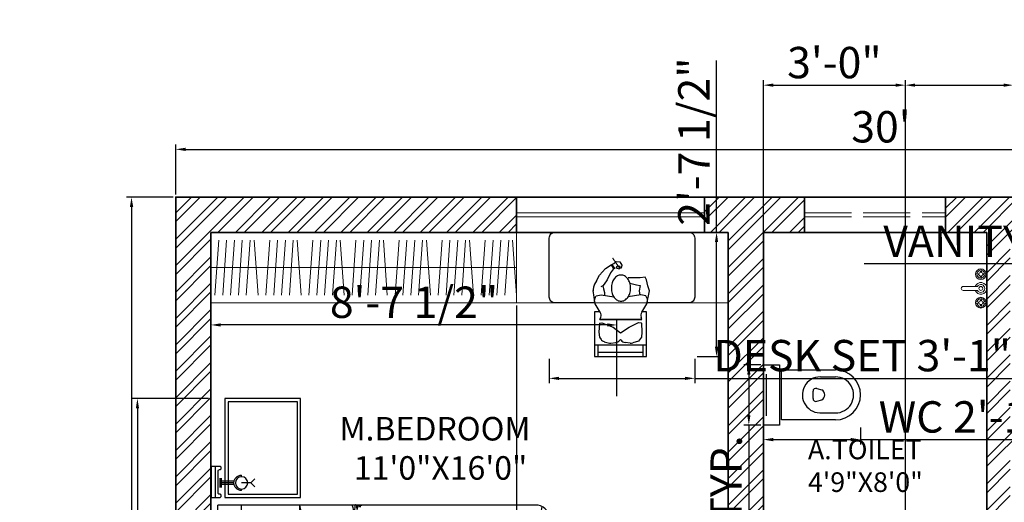
# Model space of a CAD drawing. Units: inches. Extents: x 3595 to 4516, y 2363 to 2965.
# Tile 11 of 12: x 4041 to 4293, y 2825 to 2948. Entities that reach past the tile are written whole.
import ezdxf

# ---------------------------------------------------------------- set-up
doc = ezdxf.new("R2010")
doc.units = ezdxf.units.IN
doc.linetypes.add('ACAD_ISO02W100', pattern=[15, 12, -3])
for name, color, linetype, lineweight in [('A-ANNO-DIMS', 2, 'Continuous', 18), ('A-AREA-IDEN', 7, 'Continuous', 18), ('A-FLOR-CASE', 9, 'Continuous', 18), ('A-FLOR-FIXT', 8, 'Continuous', 18), ('A-FURN', 43, 'Continuous', 18), ('A-GLAZ', 4, 'Continuous', 18), ('A-GLAZ-HIGH', 4, 'ACAD_ISO02W100', 18), ('A-WALL', 7, 'Continuous', 35)]:
    doc.layers.add(name, color=color, linetype=linetype, lineweight=lineweight)
doc.layers.add('A-WALL-PATT', color=251, linetype='Continuous', lineweight=13, true_color=0x636466)
for name, color, linetype in [('CEIL', 4, 'Continuous'), ('ELEC', 4, 'Continuous'), ('FUR', 42, 'Continuous'), ('NOITHAT', 21, 'Continuous'), ('SANTEH', 7, 'Continuous'), ('wood', 26, 'Continuous')]:
    doc.layers.add(name, color=color, linetype=linetype)
doc.styles.get("Standard").update_dxf_attribs({"font": 'arial.ttf'})
doc.dimstyles.new('ISO-25', dxfattribs={"dimtxt": 8, "dimasz": 2.5, "dimexe": 1.25, "dimexo": 0.625, "dimtad": 1, "dimdec": 1, "dimlunit": 3, "dimtxsty": 'Standard', "dimcen": 2.5, "dimadec": 0, "dimazin": 0, "dimtfac": 1, "dimtdec": 1, "dimtmove": 0, "dimatfit": 3, "dimfxl": 1, "dimarcsym": 0})

# ---------------------------------------------------------------- blocks, each defined once
blk = doc.blocks.new('*D5')
at = {"layer": 'A-ANNO-DIMS', "color": 0, "lineweight": -2, "transparency": 16777216}
for p, q in [((4081.24, 2903.67), (4081.24, 2916.47)), ((4441.24, 2903.67), (4441.24, 2916.47)), ((4083.74, 2915.22), (4438.74, 2915.22))]:
    blk.add_line(p, q, dxfattribs=at)
at = {"layer": 'A-ANNO-DIMS', "color": 0, "transparency": 16777216}
for points in [[(4083.74, 2915.63), (4083.74, 2914.8), (4081.24, 2915.22)], [(4438.74, 2915.63), (4438.74, 2914.8), (4441.24, 2915.22)]]:
    blk.add_solid(points, dxfattribs=at)
at = {"layer": 'Defpoints', "color": 0, "transparency": 16777216}
for p in [(4441.24, 2915.22), (4081.24, 2903.04), (4441.24, 2903.04)]:
    blk.add_point(p, dxfattribs=at)
at = {"layer": 'A-ANNO-DIMS', "color": 0, "transparency": 16777216, "insert": (4261.24, 2919.93), "char_height": 8, "attachment_point": 5}
blk.add_mtext("30'", dxfattribs=at)
blk = doc.blocks.new('*D6')
at = {"layer": 'A-ANNO-DIMS', "color": 0, "lineweight": -2, "transparency": 16777216}
for p, q in [((4080.62, 2903.04), (4068.71, 2903.04)), ((4069.96, 2900.54), (4069.96, 2401.54)), ((4080.62, 2399.04), (4068.71, 2399.04))]:
    blk.add_line(p, q, dxfattribs=at)
at = {"layer": 'A-ANNO-DIMS', "color": 0, "transparency": 16777216}
for points in [[(4069.55, 2900.54), (4070.38, 2900.54), (4069.96, 2903.04)], [(4069.55, 2401.54), (4070.38, 2401.54), (4069.96, 2399.04)]]:
    blk.add_solid(points, dxfattribs=at)
at = {"layer": 'Defpoints', "color": 0, "transparency": 16777216}
for p in [(4081.24, 2903.04), (4069.96, 2399.04), (4081.24, 2399.04)]:
    blk.add_point(p, dxfattribs=at)
at = {"layer": 'A-ANNO-DIMS', "color": 0, "transparency": 16777216, "insert": (4065.32, 2651.04), "char_height": 8, "attachment_point": 5, "rotation": 90}
blk.add_mtext("42'", dxfattribs=at)
blk = doc.blocks.new('*X14')
at = {"color": 0}
for p, q in [((3155.9, 8182.9), (3155.9, 8182.9)), ((3147.8, 8143.4), (3147.8, 8143.4)), ((3283, 8049.6), (3283, 8049.6)), ((3209.5, 8023.9), (3209.5, 8023.9)), ((3251.6, 7997), (3251.6, 7997)), ((3154.1, 7950.7), (3154.1, 7950.7))]:
    blk.add_line(p, q, dxfattribs=at)
blk = doc.blocks.new('*X13')
at = {"color": 0}
for p, q in [((3155.9, 8182.9), (3155.9, 8182.9)), ((3139.8, 7939.7), (3139.8, 7939.7))]:
    blk.add_line(p, q, dxfattribs=at)
blk = doc.blocks.new('*X12')
at = {"color": 0}
for p, q in [((3155.9, 8182.9), (3155.9, 8182.9)), ((3139.8, 7939.7), (3139.8, 7939.7))]:
    blk.add_line(p, q, dxfattribs=at)
blk = doc.blocks.new('*X11')
at = {"color": 0}
for p, q in [((3163, 7776.2), (3163, 7776.2)), ((3422.2, 7761.3), (3422.2, 7761.3)), ((3236.2, 7675.7), (3236.2, 7675.7)), ((3244.3, 7698.6), (3244.3, 7698.6)), ((3340.3, 7689.4), (3340.3, 7689.4))]:
    blk.add_line(p, q, dxfattribs=at)
blk = doc.blocks.new('BED1')
for p, q in [((0, -1000), (0, 800)), ((150, 800), (0, 800)), ((150, 800), (150, -1000)), ((2058.7, 800), (150, 800)), ((528, 800), (528, -1000)), ((211.8, 614.9), (277.5, 585.4)), ((2537.2, 404.9), (2237.2, 404.9)), ((2187.2, 354.9), (2187.2, -545.1)), ((2587.2, -545.1), (2587.2, 354.9)), ((2566.3, 178.5), (2565.2, 177.4)), ((2582, 188.1), (2565.4, 174.8)), ((2565.4, 174.8), (2585.7, 165.4)), ((2566.3, -296.8), (2565.2, -297.9)), ((2582, -287.1), (2565.4, -300.5)), ((2565.4, -300.5), (2585.7, -309.9)), ((2237.2, -595.1), (2537.2, -595.1)), ((150, -1000), (0, -1000)), ((150, -1000), (2063.5, -1000))]:
    blk.add_line(p, q)
for points in [[(934, 797.9), (930.9, 797.7), (928.3, 797.4), (926.3, 796.9), (924.9, 796.3), (923.8, 795.6), (923.1, 794.8), (922.7, 793.8), (922.5, 792.7), (922.4, 791.5), (922.5, 790.3), (922.6, 789.2), (922.6, 788.3), (922.6, 787.6), (922.4, 787.3), (922, 787.4), (921.4, 787.9), (920.6, 788.9), (919.5, 790.2), (918.4, 791.6), (917.1, 793.1), (915.9, 794.6), (914.6, 796), (913.3, 797.1), (912.2, 797.9), (911.1, 798.3), (910.1, 798.4), (909.2, 798), (908.3, 797.1), (907.5, 795.8), (906.8, 793.9), (906, 791.4), (905.4, 788.5), (904.8, 785.2), (904.2, 781.7), (903.7, 778.4), (903.2, 775.4), (902.8, 772.9), (902.5, 771.3), (902.3, 770.6), (902.1, 771.2), (902, 772.8), (901.8, 775.2), (901.7, 778.1), (901.5, 781.5), (901.2, 785), (900.8, 788.4), (900.2, 791.5), (899.5, 794.1), (898.6, 796.2), (897.6, 797.9), (896.5, 799.2), (895.3, 800), (894.1, 800.5), (893, 800.7), (891.9, 800.5), (890.9, 800.1), (890, 799), (889.1, 797.1), (888.3, 794), (887.6, 789.3), (886.9, 782.9), (886.2, 774.2), (885.5, 763.1), (884.8, 749.5), (884.2, 734.2), (883.6, 718.3), (883, 702.8), (882.5, 688.8), (882, 677.5), (881.7, 669.8), (881.5, 666.9), (881.3, 669.4), (881.3, 676.7), (881.3, 687.8), (881.2, 701.5), (881.1, 716.8), (880.8, 732.6), (880.2, 748), (879.4, 761.8), (878.3, 773.2), (876.9, 782.2), (875.1, 789.2), (872.9, 794.4), (870.3, 798), (869, 799)], [(2150, -913.5), (2150, 723.2)], [(2327.6, 182.3), (2530, 185.9), (2550.8, 181.9), (2561.7, 179), (2566, 176.7), (2566.9, 174.4), (2566.3, 171.9), (2562, 169.2), (2550.3, 166.5), (2527.7, 163.9), (2490.6, 161.8), (2345.5, 160.2), (2317.8, 158.5)], [(494.7, 3.1), (458.9, 95.3)], [(2149.7, -259.9), (2150, -268.4), (2150.1, -274.1), (2150.1, -278.1), (2150, -281.4), (2149.8, -284), (2149.5, -286.1), (2149.1, -287.8), (2148.7, -289), (2148.1, -289.9), (2147.4, -290.5), (2146.6, -290.8), (2145.6, -291), (2144.6, -291), (2143.6, -291), (2142.7, -290.9), (2141.9, -290.9), (2141.4, -290.9), (2141.1, -291), (2141.2, -291.4), (2141.7, -291.9), (2142.5, -292.6), (2143.5, -293.4), (2144.7, -294.4), (2146, -295.4), (2147.2, -296.5), (2148.4, -297.6), (2149.3, -298.6), (2150, -299.6), (2150.3, -300.5), (2150.4, -301.3), (2150, -302.1), (2149.3, -302.8), (2148.2, -303.5), (2146.6, -304.1), (2144.6, -304.7), (2142.1, -305.2), (2139.3, -305.7), (2136.5, -306.2), (2133.7, -306.6), (2131.2, -307), (2129.2, -307.3), (2127.8, -307.6), (2127.3, -307.8), (2127.7, -308), (2129, -308.1), (2131, -308.2), (2133.5, -308.3), (2136.3, -308.5), (2139.2, -308.7), (2142, -309), (2144.6, -309.5), (2146.8, -310.1), (2148.6, -310.9), (2150, -311.7), (2151, -312.7), (2151.7, -313.6), (2152.1, -314.6), (2152.3, -315.6), (2152.2, -316.5), (2151.8, -317.3), (2150.9, -318.1), (2149.3, -318.8), (2146.7, -319.4), (2142.8, -320), (2137.4, -320.6), (2130.2, -321.2), (2121, -321.8), (2109.7, -322.3), (2096.9, -322.9), (2083.6, -323.4), (2070.7, -323.9), (2059.1, -324.3), (2049.6, -324.7), (2043.2, -325), (2040.8, -325.2), (2042.9, -325.3), (2049, -325.3), (2058.2, -325.3), (2069.6, -325.4), (2082.3, -325.5), (2095.6, -325.8), (2108.4, -326.2), (2119.9, -326.8), (2129.4, -327.8), (2136.9, -329), (2142.7, -330.5), (2147, -332.3), (2150, -334.4), (2150.9, -335.6)], [(2246.5, -294.4), (2530, -289.4), (2550.8, -293.4), (2561.7, -296.3), (2566, -298.6), (2566.9, -300.8), (2566.3, -303.4), (2562, -306.1), (2550.3, -308.8), (2527.7, -311.3), (2490.6, -313.5), (2345.5, -315), (2238.6, -321.8)], [(1733.7, -998.3), (1731.1, -998.1), (1729, -997.8), (1727.4, -997.4), (1726.1, -997), (1725.2, -996.4), (1724.7, -995.7), (1724.3, -994.8), (1724.1, -993.9), (1724.1, -992.9), (1724.1, -991.9), (1724.2, -991), (1724.2, -990.2), (1724.2, -989.7), (1724.1, -989.4), (1723.8, -989.5), (1723.2, -990), (1722.5, -990.8), (1721.7, -991.8), (1720.7, -993), (1719.7, -994.3), (1718.6, -995.5), (1717.5, -996.6), (1716.5, -997.6), (1715.5, -998.3), (1714.6, -998.6), (1713.8, -998.6), (1713, -998.3), (1712.3, -997.6), (1711.7, -996.5), (1711, -994.9), (1710.4, -992.9), (1709.9, -990.4), (1709.4, -987.6), (1708.9, -984.8), (1708.5, -982), (1708.1, -979.5), (1707.8, -977.4), (1707.5, -976.1), (1707.3, -975.5), (1707.1, -976), (1707, -977.3), (1706.9, -979.3), (1706.8, -981.8), (1706.7, -984.6), (1706.4, -987.5), (1706.1, -990.3), (1705.6, -992.9), (1705, -995.1), (1704.2, -996.9), (1703.4, -998.3), (1702.4, -999.3), (1701.5, -1000), (1700.5, -1000.4), (1699.6, -1000.6), (1698.7, -1000.4), (1697.8, -1000.1), (1697, -999.2), (1696.3, -997.6), (1695.7, -995), (1695.1, -991.1), (1694.5, -985.7), (1693.9, -978.5), (1693.3, -969.3), (1692.8, -957.9), (1692.2, -945.2), (1691.7, -931.9), (1691.2, -919), (1690.8, -907.4), (1690.4, -897.9), (1690.1, -891.5), (1689.9, -889.1), (1689.8, -891.2), (1689.8, -897.3), (1689.8, -906.5), (1689.7, -917.9), (1689.6, -930.6), (1689.4, -943.8), (1688.9, -956.6), (1688.3, -968.1), (1687.3, -977.6), (1686.1, -985.2), (1684.6, -991), (1682.8, -995.3), (1680.7, -998.3), (1679.6, -999.2)]]:
    blk.add_lwpolyline(points)
for points in [[(489.2, 619.6, 0.144019), (207.6, 617.9, 0.248643)], [(205.5, 619.6, 0.267769), (215.1, 582.4, -0.037739), (204.3, 21.8, 0.684696), (236.7, 5.5, -0.060702), (497.2, 0.1, -0.046649), (225.9, 3.1, -1.318436)], [(497.2, 0.1, 0.021276), (489.2, 619.6, -0.206383), (326.6, 509.4, 0.237198)], [(211.8, 12.8, 0.143972), (361.6, 262.9, 1.292232)], [(886.4, -150, -0.069098), (985, -66.5, 0.658965), (982.1, -48.7, -0.049789), (927.4, -29, -0.103757), (896.6, -5.4, 0.055725), (800.9, 83.3, -0.11866), (782.7, 104.9, 0.016811), (761.6, 143.9, 0.70791), (748.3, 144, -0.16964), (551.9, -96.6, 0.664036), (554, -110.7, 0.023706), (627, -144.7, -0.134834), (683.2, -188, 0.012748), (746.3, -267.4)], [(969.1, -259.1, 0.263265), (936.3, -236.9, -0.026108), (909.2, -233.2, 0.027613), (945.1, -234.2, -0.089259), (872.7, -120, 0.662242), (857.6, -119.3, -0.162037), (651.8, -332.7, 0.676499), (654, -354.5, -0.160513), (722.9, -401.5, 0.07473), (773.5, -450.3, -0.187721), (845.5, -559.9, 0.70791), (858.8, -561.4, -0.010003), (898.6, -497.3, -0.113819), (947.3, -450.2, 0.099539), (1032.5, -372.4, -0.173425), (1070.9, -346.4, 0.589988), (1076.2, -326.1, 0.137312), (923.9, -245.9, 0.137312)], [(205.5, -168.2, 0.267769), (215.1, -205.4, -0.037739), (204.3, -766, 0.684696), (236.7, -782.3, -0.060702), (497.2, -787.7, -0.046649), (225.9, -784.7, -1.318436)], [(489.2, -168.2, 0.144019), (207.6, -169.9, 0.248643)], [(497.2, -787.7, 0.021276), (489.2, -168.2, -0.206383), (326.6, -278.4, 0.237198)], [(1446, -733.4, -0.095039), (652.8, -1001.7)]]:
    blk.add_lwpolyline(points, format="xyb")
for centre, radius, start, end in [((3208.8, 1363.3), 2739.4, 191.86791, 206.32469), ((1608.1, 842.5), 496.3, 305.19014, 354.02057), ((2062.7, 713.7), 86.5, 0, 93.53765), ((1138.6, 793.9), 983.2, 294.60777, 358.30329), ((2237.2, 354.9), 50, 90, 180), ((2321.1, 409.7), 84.5, 185.61958, 217.13957), ((2227.5, 373.5), 32.8, 17.83305, 72.80048), ((2546.9, 373.5), 32.8, 107.19952, 162.16695), ((2453.3, 409.7), 84.5, 322.86043, 354.38042), ((2537.2, 354.9), 50, 0, 90), ((2098.7, 754.7), 1625, 193.90497, 207.81692), ((2201.9, 323.3), 34.8, 50.8413, 114.9586), ((2212.2, 381.5), 36.5, 226.80948, 258.3841), ((2572.5, 323.3), 34.8, 65.0414, 129.1587), ((2562.2, 381.5), 36.5, 281.6159, 313.19052), ((751.8, 88.7), 34.9, 336.83517, 27.72181), ((684.2, 86), 100.3, 353.675, 10.88198), ((1074.1, 198.8), 306.1, 197.86019, 241.51221), ((341.4, -277.7), 318.5, 60.71255, 115.00895), ((983.7, -79.5), 20.8, 73.79673, 130.45661), ((978.5, -68.6), 14.3, 39.7097, 85.9506), ((602.5, -324), 198.6, 43.20348, 95.05559), ((3208.8, 1363.3), 2739.4, 212.93136, 216.95099), ((981.1, -281.8), 131.1, 164.0372, 243.45361), ((980, -379), 163.4, 152.61037, 209.36102), ((3208.8, 1363.3), 2739.4, 218.63292, 229.94485), ((2098.7, 754.7), 1625, 226.58872, 246.3156), ((3402.5, -342.9), 1408.5, 182.99169, 205.68187), ((-34.4, -471.2), 376.5, 312.01178, 350.96348), ((2178, -513.5), 33, 286.18268, 338.13858), ((2237.2, -545.1), 50, 180, 270), ((2188.1, -476.2), 73, 269.45125, 322.80265), ((2271.1, -580.9), 35.8, 148.90546, 197.55407), ((2546.9, -563.8), 32.8, 197.83305, 252.80048), ((2453.3, -600), 84.5, 5.61958, 37.13957), ((2537.2, -545.1), 50, 270, 0), ((2572.5, -513.6), 34.8, 230.8413, 294.9586), ((2562.2, -571.8), 36.5, 46.80948, 78.3841), ((375.7, -807.4), 128.2, 17.40732, 88.51286), ((341.4, -1065.5), 318.5, 60.71255, 115.00895), ((1929.1, -1126), 250.5, 37.85533, 88.44053), ((2063.5, -913.5), 86.5, 270, 0)]:
    blk.add_arc(centre, radius, start, end)
for name in ['*X13', '*X12', '*X14', '*X11']:
    blk.add_blockref(name, (-2425.3, -8101.4))
blk = doc.blocks.new('APLIQ')
at = {"layer": 'ELEC'}
for p, q in [((0, 0.2), (-0.0261, 0.2261)), ((0, 0.2), (0.0261, 0.2261)), ((0, 0.2), (0, 0.14)), ((-0.05, 0.14), (-0.04, 0.14)), ((0.04, 0.14), (0.05, 0.14)), ((-0.01, 0.09), (-0.01, 0.01)), ((0, 0.09), (0, 0)), ((0.01, 0.09), (0.01, 0.01)), ((-0.03, 0.01), (0.03, 0.01)), ((-0.03, 0), (0.03, 0))]:
    blk.add_line(p, q, dxfattribs=at)
blk.add_circle((0, 0.14), 0.04, dxfattribs=at)
blk.add_arc((0, 0.14), 0.05, 180, 0, dxfattribs=at)
blk = doc.blocks.new('A$C68AE1801')
at = {"layer": 'FUR'}
for points in [[(2.5416, 3.18), (2.5416, 2.54), (2.0516, 2.54), (2.0516, 3.18)], [(2.5216, 3.16), (2.5216, 2.56), (2.0716, 2.56), (2.0716, 3.16)], [(2.5416, 0), (2.5416, 0.64), (2.0516, 0.64), (2.0516, 0)], [(2.5216, 0.02), (2.5216, 0.62), (2.0716, 0.62), (2.0716, 0.02)]]:
    blk.add_lwpolyline(points, close=True, dxfattribs=at)
at = {"layer": 'wood'}
for p, q in [((2.6057, 2.74), (2.6057, 2.54)), ((2.6057, 0.44), (2.6057, 0.64))]:
    blk.add_line(p, q, dxfattribs=at)
for points in [[(2.5657, 2.728), (2.5657, 2.732, -0.414214), (2.5737, 2.74), (2.6321, 2.74), (2.6321, 2.54), (2.5737, 2.54, -0.414214), (2.5657, 2.548), (2.5657, 2.552, -0.414214), (2.5737, 2.56), (2.5777, 2.56, 0.414214), (2.5857, 2.568), (2.5857, 2.712, 0.414214), (2.5777, 2.72), (2.5737, 2.72, -0.414214)], [(2.5657, 0.452), (2.5657, 0.448, 0.414214), (2.5737, 0.44), (2.6321, 0.44), (2.6321, 0.64), (2.5737, 0.64, 0.414214), (2.5657, 0.632), (2.5657, 0.628, 0.414214), (2.5737, 0.62), (2.5777, 0.62, -0.414214), (2.5857, 0.612), (2.5857, 0.468, -0.414214), (2.5777, 0.46), (2.5737, 0.46, 0.414214)]]:
    blk.add_lwpolyline(points, format="xyb", close=True, dxfattribs=at)
at = {"layer": 'CEIL', "rotation": 90}
blk.add_blockref('APLIQ', (2.5736, 2.634), dxfattribs=at)
at = {"layer": 'CEIL', "xscale": -1, "rotation": 90}
blk.add_blockref('APLIQ', (2.5736, 0.546), dxfattribs=at)
at = {"layer": 'FUR', "xscale": 0.001, "yscale": 0.001, "zscale": 0.001, "rotation": 180}
blk.add_blockref('BED1', (2.5872, 1.49), dxfattribs=at)
blk = doc.blocks.new('y3')
at = {"layer": 'SANTEH', "ltscale": 5}
for p, q in [((37.5, 130.7), (37.5, 520.7)), ((87.5, 410.7), (87.5, 520.7)), ((346.6, 426.1), (347.5, 520.7)), ((397.5, 520.7), (397.5, 130.7)), ((171.9, 384.5), (181.1, 421.3)), ((244.3, 357.8), (190.7, 357.8)), ((263.1, 384.5), (253.9, 421.3)), ((397.5, 130.7), (37.5, 130.7)), ((67.5, 20.7), (367.5, 20.7))]:
    blk.add_line(p, q, dxfattribs=at)
blk.add_lwpolyline([(0, 115), (435, 115), (435, 0), (0, 0), (0, 115)], dxfattribs=at)
for centre, radius, start, end in [((217.5, 520.7), 180, 0, 180), ((217.5, 520.7), 130, 359.15795, 180), ((217.5, 399.9), 42.2, 30.52342, 149.47658), ((217.5, 410.7), 130, 180, 5.98548), ((190.7, 377.8), 20, 160.50385, 270), ((244.3, 377.8), 20, 270, 19.49615)]:
    blk.add_arc(centre, radius, start, end, dxfattribs=at)
blk = doc.blocks.new('Faucet - Bathroom top')
for p, q in [((-4.107, 0.125), (-4.375, 0.125)), ((-3.75, 0.4788), (-3.75, 0.75)), ((-3.5, 0.482), (-3.5, 0.75)), ((-3.1461, 0.125), (-2.875, 0.125)), ((3.143, 0.125), (2.875, 0.125)), ((3.5, 0.4788), (3.5, 0.75)), ((3.75, 0.482), (3.75, 0.75)), ((4.1039, 0.125), (4.375, 0.125)), ((-4.1039, -0.125), (-4.375, -0.125)), ((-3.75, -0.4821), (-3.75, -0.75)), ((-3.5, -0.4789), (-3.5, -0.75)), ((-3.143, -0.125), (-2.875, -0.125)), ((-0.5, -0.8639), (-0.5, -4.5)), ((0.5, -4.5), (0.5, -0.8631)), ((3.1461, -0.125), (2.875, -0.125)), ((3.5, -0.4821), (3.5, -0.75)), ((3.75, -0.4789), (3.75, -0.75)), ((4.107, -0.125), (4.375, -0.125))]:
    blk.add_line(p, q)
for centre, radius in [((-3.625, 0), 1.375), ((-4.625, 0), 0.2795), ((-3.625, 0), 0.5), ((-3.625, 1), 0.2795), ((-2.625, 0), 0.2795), ((0, 0), 0.5), ((3.625, 0), 1.375), ((2.625, 0), 0.2795), ((3.625, 0), 0.5), ((3.625, 1), 0.2795), ((4.625, 0), 0.2795), ((-3.625, -1), 0.2795), ((3.625, -1), 0.2795)]:
    blk.add_circle(centre, radius)
for centre, radius, start, end in [((-3.625, 0), 1, 105.2407, 164.2093), ((-3.625, 0), 1, 16.44125, 74.07887), ((0, 0), 1.5, 289.6514, 250.3603), ((0, 0), 1, 300.3431, 239.7554), ((3.625, 0), 1, 106.12, 164.0884), ((3.625, 0), 1, 16.23422, 73.90469), ((-3.625, 0), 1, 196.2342, 253.9047), ((-3.625, 0), 1, 286.12, 344.0884), ((3.625, 0), 1, 196.4413, 254.0789), ((3.625, 0), 1, 285.2407, 344.2093), ((0, -4.5), 0.5, 180, 0)]:
    blk.add_arc(centre, radius, start, end)
blk = doc.blocks.new('A$C15161FA2')
at = {"layer": 'NOITHAT'}
for p, q in [((659, 1027), (725, 1070)), ((725, 1070), (749, 1026)), ((729, 1062), (733, 1074)), ((733, 1074), (763, 1027)), ((553, 883), (587, 952)), ((587, 952), (659, 1027)), ((716, 977), (676, 896)), ((749, 1026), (716, 977)), ((763, 1027), (747, 1020)), ((627, 825), (602, 814)), ((643, 847), (627, 825)), ((676, 896), (643, 847)), ((537, 615), (514, 772)), ((536, 687), (548, 709)), ((548, 709), (606, 722)), ((606, 722), (754, 696)), ((1070, 722), (922, 696)), ((1128, 709), (1070, 722)), ((1140, 687), (1128, 709)), ((596, 518), (537, 615)), ((1081, 518), (1139, 615)), ((529, 522), (529, 0)), ((593, 522), (529, 522)), ((1135, 522), (1083, 522)), ((1135, 0), (1135, 522)), ((586, 386), (580, 283)), ((589, 388), (613, 393)), ((593, 432), (602, 458)), ((1083, 432), (593, 432)), ((593, 432), (1083, 432)), ((613, 393), (748, 341)), ((935, 341), (1044, 399)), ((1044, 399), (1075, 393)), ((1083, 432), (1074, 458)), ((1077, 391), (1083, 283)), ((580, 283), (587, 225)), ((748, 341), (832, 277)), ((832, 277), (935, 341)), ((1083, 283), (1077, 225)), ((529, 135), (1135, 135)), ((568, 135), (568, 0)), ((587, 225), (605, 200)), ((642, 173), (688, 159)), ((718, 157), (777, 164)), ((824, 190), (832, 200)), ((839, 190), (832, 200)), ((945, 157), (886, 164)), ((1044, 180), (975, 159)), ((1077, 225), (1044, 180)), ((1093, 135), (1093, 0)), ((568, 52), (1093, 52)), ((529, 0), (1135, 0))]:
    blk.add_line(p, q, dxfattribs=at)
for points in [[(0, 694), (0, 1384, -0.414214), (67, 1451), (1634, 1451, -0.414214), (1700, 1384), (1700, 694, -0.414214), (1634, 627), (1150, 627, -0.478936)], [(521, 627), (67, 627, -0.414214), (0, 694)]]:
    blk.add_lwpolyline(points, format="xyb", dxfattribs=at)
at = {"layer": 'NOITHAT', "const_width": 14}
blk.add_lwpolyline([(825, 1029), (740, 1151)], dxfattribs=at)
at = {"layer": 'NOITHAT'}
for points in [[(733, 1074), (756, 1086), (782, 1109), (823, 1105), (850, 1069), (839, 1031), (827, 1032), (827, 1053), (794, 1054), (778, 1035), (820, 1026)], [(1139, 615), (1173, 767), (1154, 825), (1135, 895), (1122, 928), (1064, 921), (1006, 921), (922, 921)], [(553, 883), (529, 847), (519, 812), (514, 784), (514, 768)], [(627, 825), (635, 791), (644, 747), (644, 716)], [(941, 857), (1019, 838), (1064, 831), (1051, 767), (1057, 715)]]:
    blk.add_lwpolyline(points, dxfattribs=at)
blk.add_lwpolyline([(726, 799, 0.07405), (735, 738, 0.084801), (759, 691, 0.106336), (797, 657, 0.128955), (839, 646, 0.128955), (880, 657, 0.106336), (918, 691, 0.084801), (942, 738, 0.07405), (951, 799, 0.07405), (942, 859, 0.084801), (918, 907, 0.106336), (880, 941, 0.128955), (839, 952, 0.128955), (797, 941, 0.106336), (759, 907, 0.084801), (735, 859, 0.07405)], format="xyb", close=True, dxfattribs=at)
for centre, radius, start, end in [((598, 652), 71.4, 150.9331, 210.9765), ((1078, 652), 71.4, 329.0235, 29.0669), ((534, 481), 71.4, 341.5564, 30.9765), ((1142, 481), 71.4, 149.0235, 198.4436), ((589, 385), 2.8, 101.3044, 176.6318), ((1074, 391), 2.8, 3.3682, 78.6956), ((1074, 391), 2.8, 3.3682, 78.6956), ((663, 242), 71.4, 215.5514, 252.9054), ((709, 227), 71.4, 252.9054, 277.1215), ((768, 235), 71.4, 277.1215, 321.3261), ((895, 235), 71.4, 218.6739, 262.8785), ((954, 227), 71.4, 262.8785, 287.0946)]:
    blk.add_arc(centre, radius, start, end, dxfattribs=at)
blk = doc.blocks.new('VENT-GLAZING-36IN')
for p, q in [((0, 1), (36, 1)), ((0, 0), (36, 0))]:
    blk.add_line(p, q)
blk = doc.blocks.new('WIN-GLAZING-48IN')
for p, q in [((0, 1), (48, 1)), ((0, 0), (48, 0))]:
    blk.add_line(p, q)
blk = doc.blocks.new('*D119')
at = {"layer": 'A-ANNO-DIMS', "color": 0, "lineweight": -2, "transparency": 16777216}
for p, q in [((4089.62, 2851.64), (4070.21, 2851.64)), ((4071.46, 2849.14), (4071.46, 2728.95)), ((4089.62, 2726.45), (4070.21, 2726.45)), ((4071.46, 2726.45), (4071.46, 2590.66))]:
    blk.add_line(p, q, dxfattribs=at)
at = {"layer": 'A-ANNO-DIMS', "color": 0, "transparency": 16777216}
for points in [[(4071.05, 2849.14), (4071.88, 2849.14), (4071.46, 2851.64)], [(4071.05, 2728.95), (4071.88, 2728.95), (4071.46, 2726.45)]]:
    blk.add_solid(points, dxfattribs=at)
at = {"layer": 'Defpoints', "color": 0, "transparency": 16777216}
for p in [(4090.24, 2851.64), (4071.46, 2726.45), (4090.24, 2726.45)]:
    blk.add_point(p, dxfattribs=at)
at = {"layer": 'A-ANNO-DIMS', "color": 0, "transparency": 16777216, "insert": (4066.7, 2657.3), "char_height": 8, "attachment_point": 5, "rotation": 90}
blk.add_mtext('PRIMARY BED SET 10\'-5"', dxfattribs=at)
blk = doc.blocks.new('*D120')
at = {"layer": 'A-ANNO-DIMS', "color": 0, "lineweight": -2, "transparency": 16777216}
for p, q in [((4090.24, 2852.27), (4090.24, 2871.67)), ((4191.37, 2870.42), (4092.74, 2870.42)), ((4193.87, 2852.27), (4193.87, 2871.67))]:
    blk.add_line(p, q, dxfattribs=at)
at = {"layer": 'A-ANNO-DIMS', "color": 0, "transparency": 16777216}
for points in [[(4092.74, 2870.84), (4092.74, 2870.01), (4090.24, 2870.42)], [(4191.37, 2870.84), (4191.37, 2870.01), (4193.87, 2870.42)]]:
    blk.add_solid(points, dxfattribs=at)
at = {"layer": 'Defpoints', "color": 0, "transparency": 16777216}
for p in [(4090.24, 2870.42), (4090.24, 2851.64), (4193.87, 2851.64)]:
    blk.add_point(p, dxfattribs=at)
at = {"layer": 'A-ANNO-DIMS', "color": 0, "transparency": 16777216, "insert": (4142.06, 2875.18), "char_height": 8, "attachment_point": 5}
blk.add_mtext('8\'-7 1/2"', dxfattribs=at)
blk = doc.blocks.new('*D125')
at = {"layer": 'A-ANNO-DIMS', "color": 0, "lineweight": -2, "transparency": 16777216}
for p, q in [((4176.58, 2861.74), (4176.58, 2855.55)), ((4213.71, 2861.74), (4213.71, 2855.55)), ((4179.08, 2856.8), (4211.21, 2856.8)), ((4213.71, 2856.8), (4296.71, 2856.8))]:
    blk.add_line(p, q, dxfattribs=at)
at = {"layer": 'A-ANNO-DIMS', "color": 0, "transparency": 16777216}
for points in [[(4179.08, 2857.21), (4179.08, 2856.38), (4176.58, 2856.8)], [(4211.21, 2857.21), (4211.21, 2856.38), (4213.71, 2856.8)]]:
    blk.add_solid(points, dxfattribs=at)
at = {"layer": 'Defpoints', "color": 0, "transparency": 16777216}
for p in [(4176.58, 2862.37), (4213.71, 2862.37), (4213.71, 2856.8)]:
    blk.add_point(p, dxfattribs=at)
at = {"layer": 'A-ANNO-DIMS', "color": 0, "transparency": 16777216, "insert": (4256.46, 2861.56), "char_height": 8, "attachment_point": 5}
blk.add_mtext('DESK SET 3\'-1"', dxfattribs=at)
blk = doc.blocks.new('*D126')
at = {"layer": 'A-ANNO-DIMS', "color": 0, "lineweight": -2, "transparency": 16777216}
for p, q in [((4219.28, 2894.04), (4219.28, 2937.84)), ((4214.33, 2894.04), (4220.53, 2894.04)), ((4219.28, 2864.87), (4219.28, 2891.54)), ((4214.33, 2862.37), (4220.53, 2862.37))]:
    blk.add_line(p, q, dxfattribs=at)
at = {"layer": 'A-ANNO-DIMS', "color": 0, "transparency": 16777216}
for points in [[(4218.86, 2891.54), (4219.69, 2891.54), (4219.28, 2894.04)], [(4218.86, 2864.87), (4219.69, 2864.87), (4219.28, 2862.37)]]:
    blk.add_solid(points, dxfattribs=at)
at = {"layer": 'Defpoints', "color": 0, "transparency": 16777216}
for p in [(4213.71, 2894.04), (4219.28, 2894.04), (4213.71, 2862.37)]:
    blk.add_point(p, dxfattribs=at)
at = {"layer": 'A-ANNO-DIMS', "color": 0, "transparency": 16777216, "insert": (4214.52, 2917.19), "char_height": 8, "attachment_point": 5, "rotation": 90}
blk.add_mtext('2\'-7 1/2"', dxfattribs=at)
blk = doc.blocks.new('*D127')
at = {"layer": 'A-ANNO-DIMS', "color": 0, "lineweight": -2, "transparency": 16777216}
for p, q in [((4404.25, 2885.98), (4256.92, 2885.98)), ((4404.25, 2883.56), (4404.25, 2887.23)), ((4422.09, 2885.98), (4406.75, 2885.98)), ((4424.59, 2883.56), (4424.59, 2887.23))]:
    blk.add_line(p, q, dxfattribs=at)
at = {"layer": 'A-ANNO-DIMS', "color": 0, "transparency": 16777216}
for points in [[(4406.75, 2886.4), (4406.75, 2885.57), (4404.25, 2885.98)], [(4422.09, 2886.4), (4422.09, 2885.57), (4424.59, 2885.98)]]:
    blk.add_solid(points, dxfattribs=at)
at = {"layer": 'Defpoints', "color": 0, "transparency": 16777216}
for p in [(4404.25, 2885.98), (4404.25, 2882.93), (4424.59, 2882.93)]:
    blk.add_point(p, dxfattribs=at)
at = {"layer": 'A-ANNO-DIMS', "color": 0, "transparency": 16777216, "insert": (4329.34, 2890.75), "char_height": 8, "attachment_point": 5}
blk.add_mtext('VANITY SEAT 1\'-8 1/2" TYP.', dxfattribs=at)
blk = doc.blocks.new('*D131')
at = {"layer": 'A-ANNO-DIMS', "color": 0, "lineweight": -2, "transparency": 16777216}
for p, q in [((4231.24, 2844.27), (4231.24, 2839.92)), ((4256.04, 2844.27), (4256.04, 2839.92)), ((4233.74, 2841.17), (4253.54, 2841.17)), ((4256.04, 2841.17), (4330.6, 2841.17))]:
    blk.add_line(p, q, dxfattribs=at)
at = {"layer": 'A-ANNO-DIMS', "color": 0, "transparency": 16777216}
for points in [[(4233.74, 2841.59), (4233.74, 2840.75), (4231.24, 2841.17)], [(4253.54, 2841.59), (4253.54, 2840.75), (4256.04, 2841.17)]]:
    blk.add_solid(points, dxfattribs=at)
at = {"layer": 'Defpoints', "color": 0, "transparency": 16777216}
for p in [(4231.24, 2844.89), (4256.04, 2844.89), (4256.04, 2841.17)]:
    blk.add_point(p, dxfattribs=at)
at = {"layer": 'A-ANNO-DIMS', "color": 0, "transparency": 16777216, "insert": (4294.57, 2845.93), "char_height": 8, "attachment_point": 5}
blk.add_mtext('WC 2\'-1" TYP.', dxfattribs=at)
blk = doc.blocks.new('*D132')
at = {"layer": 'A-ANNO-DIMS', "color": 0, "lineweight": -2, "transparency": 16777216}
for p, q in [((4230.62, 2860.28), (4226.27, 2860.28)), ((4227.52, 2857.78), (4227.52, 2847.39)), ((4230.62, 2844.89), (4226.27, 2844.89)), ((4227.52, 2844.89), (4227.52, 2774.49))]:
    blk.add_line(p, q, dxfattribs=at)
at = {"layer": 'A-ANNO-DIMS', "color": 0, "transparency": 16777216}
for points in [[(4227.11, 2857.78), (4227.94, 2857.78), (4227.52, 2860.28)], [(4227.11, 2847.39), (4227.94, 2847.39), (4227.52, 2844.89)]]:
    blk.add_solid(points, dxfattribs=at)
at = {"layer": 'Defpoints', "color": 0, "transparency": 16777216}
for p in [(4231.24, 2860.28), (4227.52, 2844.89), (4231.24, 2844.89)]:
    blk.add_point(p, dxfattribs=at)
at = {"layer": 'A-ANNO-DIMS', "color": 0, "transparency": 16777216, "insert": (4222.76, 2808.44), "char_height": 8, "attachment_point": 5, "rotation": 90}
blk.add_mtext('1\'-3 1/2" TYP.', dxfattribs=at)
blk = doc.blocks.new('*D163')
at = {"layer": 'A-ANNO-DIMS', "color": 0, "lineweight": -2, "transparency": 16777216}
for p, q in [((4267.47, 2626.41), (4267.47, 2932.84)), ((4295.03, 2624.44), (4295.03, 2932.84)), ((4269.97, 2931.59), (4292.53, 2931.59)), ((4295.03, 2931.59), (4338.82, 2931.59))]:
    blk.add_line(p, q, dxfattribs=at)
at = {"layer": 'A-ANNO-DIMS', "color": 0, "transparency": 16777216}
for points in [[(4269.97, 2932.01), (4269.97, 2931.18), (4267.47, 2931.59)], [(4292.53, 2932.01), (4292.53, 2931.18), (4295.03, 2931.59)]]:
    blk.add_solid(points, dxfattribs=at)
at = {"layer": 'Defpoints', "color": 0, "transparency": 16777216}
for p in [(4295.03, 2931.59), (4267.47, 2625.78), (4295.03, 2623.82)]:
    blk.add_point(p, dxfattribs=at)
at = {"layer": 'A-ANNO-DIMS', "color": 0, "transparency": 16777216, "insert": (4318.18, 2936.36), "char_height": 8, "attachment_point": 5}
blk.add_mtext('2\'-3 1/2"', dxfattribs=at)
blk = doc.blocks.new('*D167')
at = {"layer": 'A-ANNO-DIMS', "color": 0, "lineweight": -2, "transparency": 16777216}
for p, q in [((4231.24, 2606.67), (4231.24, 2932.84)), ((4267.47, 2626.41), (4267.47, 2932.84)), ((4233.74, 2931.59), (4264.97, 2931.59))]:
    blk.add_line(p, q, dxfattribs=at)
at = {"layer": 'A-ANNO-DIMS', "color": 0, "transparency": 16777216}
for points in [[(4233.74, 2932.01), (4233.74, 2931.18), (4231.24, 2931.59)], [(4264.97, 2932.01), (4264.97, 2931.18), (4267.47, 2931.59)]]:
    blk.add_solid(points, dxfattribs=at)
at = {"layer": 'Defpoints', "color": 0, "transparency": 16777216}
for p in [(4267.47, 2931.59), (4267.47, 2625.78), (4231.24, 2606.04)]:
    blk.add_point(p, dxfattribs=at)
at = {"layer": 'A-ANNO-DIMS', "color": 0, "transparency": 16777216, "insert": (4249.36, 2936.31), "char_height": 8, "attachment_point": 5}
blk.add_mtext('3\'-0"', dxfattribs=at)
blk = doc.blocks.new('*D170')
at = {"layer": 'A-ANNO-DIMS', "color": 0, "lineweight": -2, "transparency": 16777216}
for p, q in [((4090.24, 2875.42), (4090.24, 2369.24)), ((4168.24, 2875.42), (4168.24, 2369.24)), ((4092.74, 2370.49), (4165.74, 2370.49))]:
    blk.add_line(p, q, dxfattribs=at)
at = {"layer": 'A-ANNO-DIMS', "color": 0, "transparency": 16777216}
for points in [[(4092.74, 2370.91), (4092.74, 2370.08), (4090.24, 2370.49)], [(4165.74, 2370.91), (4165.74, 2370.08), (4168.24, 2370.49)]]:
    blk.add_solid(points, dxfattribs=at)
at = {"layer": 'Defpoints', "color": 0, "transparency": 16777216}
for p in [(4090.24, 2876.04), (4168.24, 2876.04), (4168.24, 2370.49)]:
    blk.add_point(p, dxfattribs=at)
at = {"layer": 'A-ANNO-DIMS', "color": 0, "transparency": 16777216, "insert": (4129.24, 2375.2), "char_height": 8, "attachment_point": 5}
blk.add_mtext('6\'-6"', dxfattribs=at)

msp = doc.modelspace()

# ---------------------------------------------------------------- hatches: boundary and pattern name
at = {"layer": 'A-WALL-PATT'}
h = msp.add_hatch(dxfattribs=at)
h.set_pattern_fill('ANSI32', color=256, scale=0.5)
h.set_pattern_definition([(45, (441.351, 0), (-3.367596, 3.367596), []), (45, (443.596, 0), (-3.367596, 3.367596), [])])
h.paths.add_polyline_path([(4081.24, 2756.04), (4090.24, 2756.04), (4090.24, 2894.04), (4168.24, 2894.04), (4168.24, 2903.04), (4081.24, 2903.04)])
h.paths.add_polyline_path([(4216.24, 2903.04), (4216.24, 2894.04), (4222.24, 2894.04), (4222.24, 2792.04), (4231.24, 2792.04), (4231.24, 2894.04), (4241.74, 2894.04), (4241.74, 2903.04)])
h.paths.add_polyline_path([(4324.24, 2894.04), (4324.24, 2903.04), (4277.74, 2903.04), (4277.74, 2894.04), (4288.24, 2894.04), (4288.24, 2798.04), (4261.24, 2798.04), (4261.24, 2792.04), (4288.24, 2792.04), (4288.24, 2756.04), (4222.24, 2756.04), (4222.24, 2702.04), (4219.24, 2702.04), (4219.24, 2693.04), (4241.74, 2693.04), (4241.74, 2702.04), (4231.24, 2702.04), (4231.24, 2750.04), (4288.24, 2750.04), (4288.24, 2702.04), (4277.74, 2702.04), (4277.74, 2693.04), (4393.24, 2693.04), (4393.24, 2702.04), (4294.24, 2702.04), (4294.24, 2840.04), (4396.24, 2840.04), (4396.24, 2846.04), (4294.24, 2846.04), (4294.24, 2894.04)])
h.paths.add_polyline_path([(4390.24, 2894.04), (4390.24, 2876.04), (4396.24, 2876.04), (4396.24, 2894.04), (4432.24, 2894.04), (4432.24, 2795.04), (4441.24, 2795.04), (4441.24, 2903.04), (4360.24, 2903.04), (4360.24, 2894.04)])
h.paths.add_polyline_path([(4090.24, 2693.04), (4183.24, 2693.04), (4183.24, 2702.04), (4090.24, 2702.04), (4090.24, 2708.04), (4081.24, 2708.04), (4081.24, 2673.54), (4090.24, 2673.54)])
h.paths.add_polyline_path([(4090.24, 2600.04), (4183.24, 2600.04), (4183.24, 2606.04), (4090.24, 2606.04), (4090.24, 2625.54), (4081.24, 2625.54), (4081.24, 2561.04), (4090.24, 2561.04)])
h.paths.add_polyline_path([(4081.24, 2399.04), (4231.24, 2399.04), (4231.24, 2405.04), (4090.24, 2405.04), (4090.24, 2477.04), (4180.24, 2477.04), (4180.24, 2486.04), (4090.24, 2486.04), (4090.24, 2525.04), (4081.24, 2525.04)])
h.paths.add_polyline_path([(4231.24, 2486.04), (4231.24, 2606.04), (4219.24, 2606.04), (4219.24, 2600.04), (4222.24, 2600.04), (4222.24, 2486.04), (4216.24, 2486.04), (4216.24, 2477.04), (4273.24, 2477.04), (4273.24, 2486.04)])
h.paths.add_polyline_path([(4339.24, 2486.04), (4339.24, 2477.04), (4381.24, 2477.04), (4381.24, 2486.04)])
h.paths.add_polyline_path([(4432.24, 2486.04), (4429.24, 2486.04), (4429.24, 2477.04), (4441.24, 2477.04), (4441.24, 2511.54), (4432.24, 2511.54)])
h.paths.add_polyline_path([(4432.24, 2571.54), (4441.24, 2571.54), (4441.24, 2607.54), (4432.24, 2607.54)])
h.paths.add_polyline_path([(4441.24, 2747.04), (4432.24, 2747.04), (4432.24, 2702.04), (4429.24, 2702.04), (4429.24, 2693.04), (4432.24, 2693.04), (4432.24, 2667.54), (4441.24, 2667.54)])

# ---------------------------------------------------------------- linework, layer by layer
at = {"layer": 'A-FLOR-CASE'}
for p, q in [((4168.24, 2894.04), (4168.24, 2876.04)), ((4092.24, 2892.04), (4091.24, 2878.04)), ((4094.24, 2892.04), (4093.24, 2878.04)), ((4096.24, 2892.04), (4095.24, 2878.04)), ((4098.24, 2892.04), (4097.24, 2878.04)), ((4100.24, 2892.04), (4099.24, 2878.04)), ((4101.24, 2892.04), (4102.24, 2878.04)), ((4105.24, 2892.04), (4104.24, 2878.04)), ((4107.24, 2892.04), (4106.24, 2878.04)), ((4109.24, 2892.04), (4108.24, 2878.04)), ((4111.24, 2892.04), (4110.24, 2878.04)), ((4112.24, 2892.04), (4113.24, 2878.04)), ((4116.24, 2892.04), (4115.24, 2878.04)), ((4118.24, 2892.04), (4117.24, 2878.04)), ((4120.24, 2892.04), (4119.24, 2878.04)), ((4122.24, 2892.04), (4121.24, 2878.04)), ((4123.24, 2892.04), (4124.24, 2878.04)), ((4127.24, 2892.04), (4126.24, 2878.04)), ((4129.24, 2892.04), (4128.24, 2878.04)), ((4131.24, 2892.04), (4130.24, 2878.04)), ((4133.24, 2892.04), (4132.24, 2878.04)), ((4134.24, 2892.04), (4135.24, 2878.04)), ((4138.24, 2892.04), (4137.24, 2878.04)), ((4140.24, 2892.04), (4139.24, 2878.04)), ((4142.24, 2892.04), (4141.24, 2878.04)), ((4144.24, 2892.04), (4143.24, 2878.04)), ((4145.24, 2892.04), (4146.24, 2878.04)), ((4149.24, 2892.04), (4148.24, 2878.04)), ((4151.24, 2892.04), (4150.24, 2878.04)), ((4153.24, 2892.04), (4152.24, 2878.04)), ((4155.24, 2892.04), (4154.24, 2878.04)), ((4156.24, 2892.04), (4157.24, 2878.04)), ((4160.24, 2892.04), (4159.24, 2878.04)), ((4162.24, 2892.04), (4161.24, 2878.04)), ((4164.24, 2892.04), (4163.24, 2878.04)), ((4166.24, 2892.04), (4165.24, 2878.04)), ((4167.24, 2892.04), (4168.24, 2878.04)), ((4168.24, 2885.04), (4090.24, 2885.04)), ((4090.24, 2876.04), (4222.24, 2876.04))]:
    msp.add_line(p, q, dxfattribs=at)
at = {"layer": 'A-WALL'}
for p, q in [((4168.24, 2894.04), (4168.24, 2903.04)), ((4216.24, 2894.04), (4216.24, 2903.04)), ((4241.74, 2894.04), (4241.74, 2903.04)), ((4277.74, 2894.04), (4277.74, 2903.04)), ((4090.24, 2894.04), (4222.24, 2894.04)), ((4090.24, 2702.04), (4090.24, 2894.04)), ((4222.24, 2792.04), (4222.24, 2894.04)), ((4231.24, 2894.04), (4288.24, 2894.04)), ((4231.24, 2792.04), (4231.24, 2894.04)), ((4288.24, 2798.04), (4288.24, 2894.04))]:
    msp.add_line(p, q, dxfattribs=at)
msp.add_lwpolyline([(4231.24, 2399.04), (4081.24, 2399.04), (4081.24, 2903.04), (4441.24, 2903.04), (4441.24, 2477.04)], dxfattribs=at)

# ---------------------------------------------------------------- block references
at = {"layer": 'A-FLOR-FIXT', "rotation": 270}
msp.add_blockref('Faucet - Bathroom top', (4286.74, 2879.74), dxfattribs=at)
at = {"layer": 'A-FLOR-FIXT', "xscale": 0.0353848906415677, "yscale": 0.0353848906415677, "zscale": 0.0353848906415677, "rotation": 270}
msp.add_blockref('y3', (4231.24, 2860.28), dxfattribs=at)
at = {"layer": 'A-FURN', "xscale": 0.021836888786069, "yscale": 0.021836888786069, "zscale": 0.021836888786069}
msp.add_blockref('A$C15161FA2', (4176.58, 2862.37), dxfattribs=at)
at = {"layer": 'A-FURN', "xscale": 39.3701, "yscale": 39.3701, "zscale": 39.3701, "rotation": 180}
msp.add_blockref('A$C68AE1801', (4193.87, 2851.64), dxfattribs=at)
at = {"layer": 'A-GLAZ'}
msp.add_blockref('WIN-GLAZING-48IN', (4168.24, 2898.04), dxfattribs=at)
at = {"layer": 'A-GLAZ-HIGH'}
msp.add_blockref('VENT-GLAZING-36IN', (4241.74, 2898.04), dxfattribs=at)

# ---------------------------------------------------------------- texts
at = {"layer": 'A-AREA-IDEN', "attachment_point": 1}
for s, insert, char_height in [('{\\fTimes New Roman|b0|i0|c0|p18;M.BEDROOM\\P  11\'0"X16\'0"}', (4123.04, 2846.95), 6), ('{\\fTimes New Roman|b0|i0|c0|p18;A.TOILET\\P4\'9"X8\'0"}', (4242.62, 2841.16), 5)]:
    msp.add_mtext_dynamic_manual_height_columns(s, width=67.3508, gutter_width=12.5, heights=[0], dxfattribs=dict(at, insert=insert, char_height=char_height))

# ---------------------------------------------------------------- dimensions: what is measured, and where the dimension line sits
at = {"layer": 'A-ANNO-DIMS'}
for base, p1, p2, override, picture, middle in [((4295.03, 2931.59), (4267.47, 2625.78), (4295.03, 2623.82), {"dimdec": 1, "dimlfac": 1, "dimrnd": 0, "dimzin": 1, "dimdsep": 46, "dimlunit": 4, "dimfrac": 2}, '*D163', (4318.18, 2936.36)), ((4267.47, 2931.59), (4231.24, 2606.04), (4267.47, 2625.78), {"dimdec": 1, "dimlfac": 1, "dimrnd": 0, "dimzin": 1, "dimdsep": 46, "dimlunit": 4, "dimfrac": 2}, '*D167', (4249.36, 2936.31)), ((4441.24, 2915.22), (4081.24, 2903.04), (4441.24, 2903.04), {"dimclrd": 0, "dimclre": 0, "dimclrt": 0}, '*D5', (4261.24, 2919.93)), ((4168.24, 2370.49), (4090.24, 2876.04), (4168.24, 2876.04), {"dimdec": 1, "dimlfac": 1, "dimrnd": 0, "dimzin": 1, "dimdsep": 46, "dimlunit": 4, "dimfrac": 2}, '*D170', (4129.24, 2375.2))]:
    dim = msp.add_linear_dim(base=base, p1=p1, p2=p2, dimstyle='ISO-25', override=override, dxfattribs=at)
    dim.commit()
    dim.dimension.update_dxf_attribs({"geometry": picture, "text_midpoint": middle})
for base, p1, p2, angle, override, picture, middle in [((4219.28, 2894.04), (4213.71, 2862.37), (4213.71, 2894.04), 90, {"dimdec": 1, "dimlfac": 1, "dimrnd": 0, "dimzin": 1, "dimdsep": 46, "dimlunit": 4, "dimfrac": 2}, '*D126', (4214.52, 2917.19)), ((4069.96, 2399.04), (4081.24, 2903.04), (4081.24, 2399.04), 90, {"dimclrd": 0, "dimclre": 0, "dimclrt": 0}, '*D6', (4065.32, 2651.04)), ((4090.24, 2870.42), (4193.87, 2851.64), (4090.24, 2851.64), 180, {"dimdec": 1, "dimlfac": 1, "dimrnd": 0, "dimzin": 1, "dimdsep": 46, "dimlunit": 4, "dimfrac": 2}, '*D120', (4142.06, 2875.18))]:
    dim = msp.add_linear_dim(base=base, p1=p1, p2=p2, angle=angle, dimstyle='ISO-25', override=override, dxfattribs=at)
    dim.commit()
    dim.dimension.update_dxf_attribs({"geometry": picture, "text_midpoint": middle})
for base, p1, p2, angle, text, picture, middle in [((4404.25, 2885.98), (4424.59, 2882.93), (4404.25, 2882.93), 180, 'VANITY SEAT <> TYP.', '*D127', (4329.34, 2890.75)), ((4227.52, 2844.89), (4231.24, 2860.28), (4231.24, 2844.89), 270, '<> TYP.', '*D132', (4222.76, 2808.44)), ((4071.46, 2726.45), (4090.24, 2851.64), (4090.24, 2726.45), 270, 'PRIMARY BED SET <>', '*D119', (4066.7, 2657.3))]:
    dim = msp.add_linear_dim(base=base, p1=p1, p2=p2, angle=angle, text=text, dimstyle='ISO-25', override={"dimdec": 1, "dimlfac": 1, "dimrnd": 0, "dimzin": 1, "dimdsep": 46, "dimlunit": 4, "dimfrac": 2}, dxfattribs=at)
    dim.commit()
    dim.dimension.update_dxf_attribs({"geometry": picture, "text_midpoint": middle})
for base, p1, p2, text, picture, middle in [((4213.71, 2856.8), (4176.58, 2862.37), (4213.71, 2862.37), 'DESK SET <>', '*D125', (4256.46, 2861.56)), ((4256.04, 2841.17), (4231.24, 2844.89), (4256.04, 2844.89), 'WC <> TYP.', '*D131', (4294.57, 2845.93))]:
    dim = msp.add_linear_dim(base=base, p1=p1, p2=p2, text=text, dimstyle='ISO-25', override={"dimdec": 1, "dimlfac": 1, "dimrnd": 0, "dimzin": 1, "dimdsep": 46, "dimlunit": 4, "dimfrac": 2}, dxfattribs=at)
    dim.commit()
    dim.dimension.update_dxf_attribs({"geometry": picture, "text_midpoint": middle})

doc.saveas('drawing.dxf')
